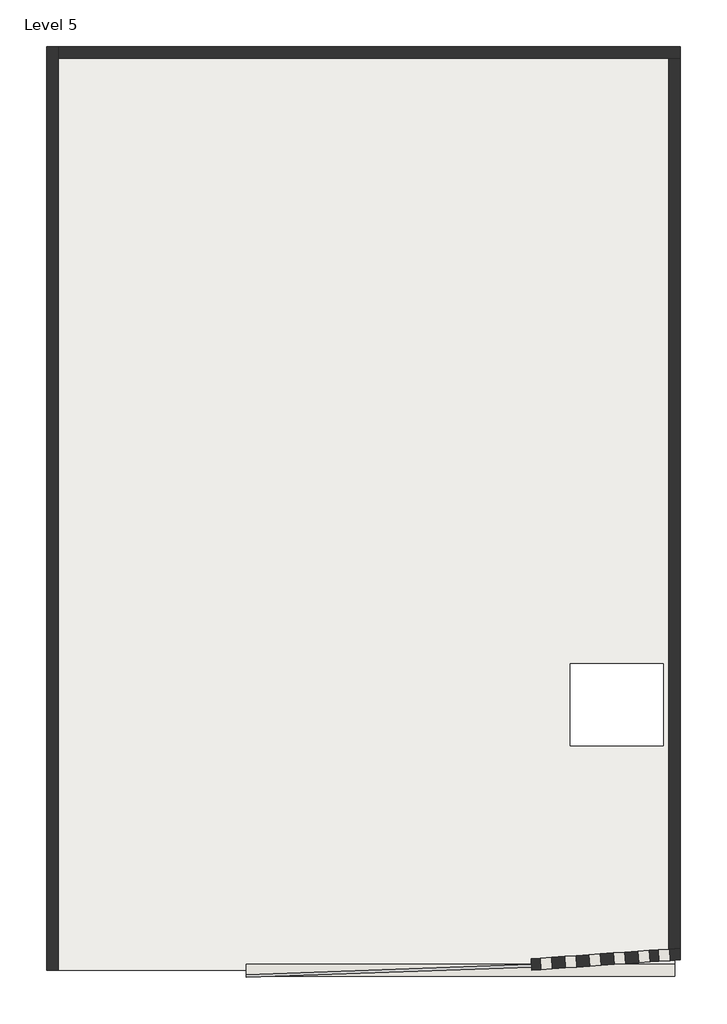
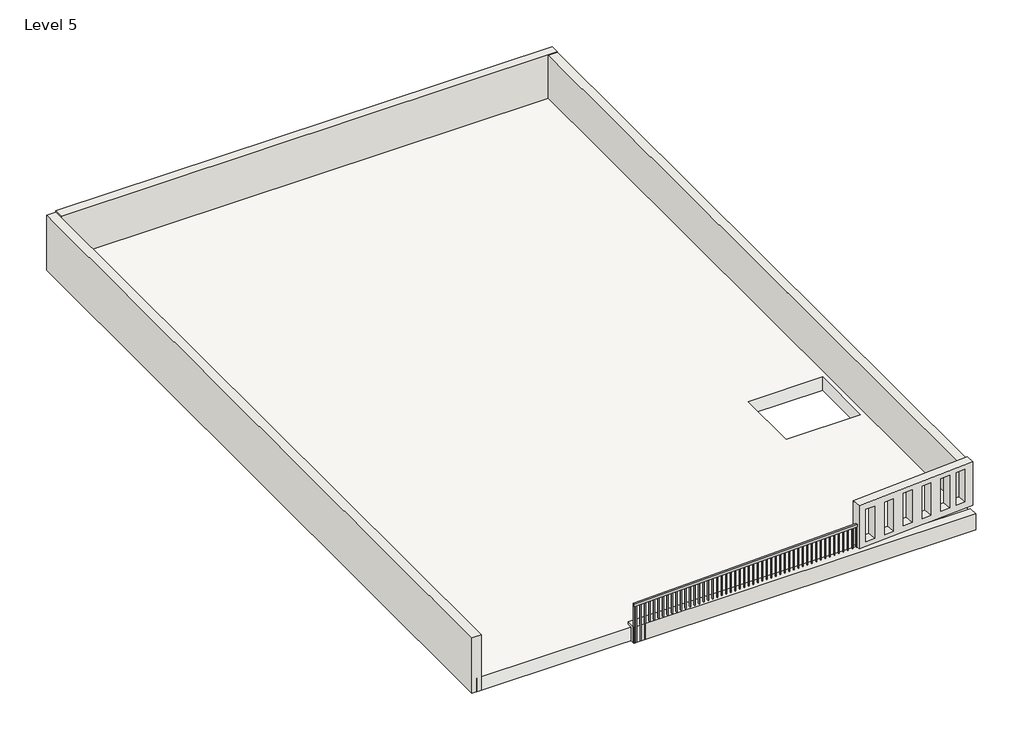
# One storey: 5 walls, 1 railing, 1 roof.
"""IFC4 building model written with IfcOpenShell, lengths in millimetres."""

from ifc_helpers import new_model, si_unit, frame, origin, place, context, project, spatial, polyline, outline, extrude, faceted_brep, element, save

model = new_model("IFC4")

# Units and contexts
model_context = context("Model", 3, world=origin())
ifc_project = project(units=[si_unit("LENGTHUNIT", "METRE", prefix="MILLI")], contexts=[model_context])

# Site, building, storey
site = spatial("IfcSite", under=ifc_project)
building = spatial("IfcBuilding", under=site)
storey = spatial("IfcBuildingStorey", under=building, Name="Level 5", Elevation=12192.0)

# Railing
placement = place(None, origin())
element("IfcRailing", 1, ObjectType="Handrail - Rectangular", at=placement, inside=storey, context=model_context, shape_type="SweptSolid", body=[
    extrude(outline(polyline([(1979.8158974, -8066.6140284), (1981.6116302, -8117.3822797), (-3046.82922, -8295.2441529), (-3048.6249528, -8244.4759015), (1979.8158974, -8066.6140284)])), frame((0.0, 0.0, 13055.6), z_axis=(0.0, 0.0, 1.0), x_axis=(1.0, 0.0, 0.0)), (0.0, 0.0, 1.0), 50.8),
    extrude(outline(polyline([(-2985.3925198, -8258.1242236), (-2984.71912, -8277.1623178), (-3003.7572143, -8277.8357176), (-3004.4306141, -8258.7976234), (-2985.3925198, -8258.1242236)])), frame((0.0, 0.0, 12192.0), z_axis=(0.0, 0.0, 1.0), x_axis=(1.0, 0.0, 0.0)), (0.0, 0.0, 1.0), 863.6),
    extrude(outline(polyline([(-2883.8560172, -8254.5327579), (-2883.1826173, -8273.5708522), (-2902.2207116, -8274.244252), (-2902.8941114, -8255.2061578), (-2883.8560172, -8254.5327579)])), frame((0.0, 0.0, 12192.0), z_axis=(0.0, 0.0, 1.0), x_axis=(1.0, 0.0, 0.0)), (0.0, 0.0, 1.0), 863.6),
    extrude(outline(polyline([(-2782.3195145, -8250.9412923), (-2781.6461147, -8269.9793866), (-2800.6842089, -8270.6527864), (-2801.3576087, -8251.6146921), (-2782.3195145, -8250.9412923)])), frame((0.0, 0.0, 12192.0), z_axis=(0.0, 0.0, 1.0), x_axis=(1.0, 0.0, 0.0)), (0.0, 0.0, 1.0), 863.6),
    extrude(outline(polyline([(-2680.7830118, -8247.3498267), (-2680.109612, -8266.3879209), (-2699.1477063, -8267.0613207), (-2699.8211061, -8248.0232265), (-2680.7830118, -8247.3498267)])), frame((0.0, 0.0, 12192.0), z_axis=(0.0, 0.0, 1.0), x_axis=(1.0, 0.0, 0.0)), (0.0, 0.0, 1.0), 863.6),
    extrude(outline(polyline([(-2579.2465091, -8243.758361), (-2578.5731093, -8262.7964553), (-2597.6112036, -8263.4698551), (-2598.2846034, -8244.4317608), (-2579.2465091, -8243.758361)])), frame((0.0, 0.0, 12192.0), z_axis=(0.0, 0.0, 1.0), x_axis=(1.0, 0.0, 0.0)), (0.0, 0.0, 1.0), 863.6),
    extrude(outline(polyline([(-2477.7100065, -8240.1668954), (-2477.0366067, -8259.2049896), (-2496.0747009, -8259.8783894), (-2496.7481007, -8240.8402952), (-2477.7100065, -8240.1668954)])), frame((0.0, 0.0, 12192.0), z_axis=(0.0, 0.0, 1.0), x_axis=(1.0, 0.0, 0.0)), (0.0, 0.0, 1.0), 863.6),
    extrude(outline(polyline([(-2376.1735038, -8236.5754297), (-2375.500104, -8255.613524), (-2394.5381982, -8256.2869238), (-2395.2115981, -8237.2488295), (-2376.1735038, -8236.5754297)])), frame((0.0, 0.0, 12192.0), z_axis=(0.0, 0.0, 1.0), x_axis=(1.0, 0.0, 0.0)), (0.0, 0.0, 1.0), 863.6),
    extrude(outline(polyline([(-2274.6370011, -8232.9839641), (-2273.9636013, -8252.0220583), (-2293.0016956, -8252.6954581), (-2293.6750954, -8233.6573639), (-2274.6370011, -8232.9839641)])), frame((0.0, 0.0, 12192.0), z_axis=(0.0, 0.0, 1.0), x_axis=(1.0, 0.0, 0.0)), (0.0, 0.0, 1.0), 863.6),
    extrude(outline(polyline([(-2173.1004985, -8229.3924984), (-2172.4270987, -8248.4305927), (-2191.4651929, -8249.1039925), (-2192.1385927, -8230.0658982), (-2173.1004985, -8229.3924984)])), frame((0.0, 0.0, 12192.0), z_axis=(0.0, 0.0, 1.0), x_axis=(1.0, 0.0, 0.0)), (0.0, 0.0, 1.0), 863.6),
    extrude(outline(polyline([(-2071.5639958, -8225.8010328), (-2070.890596, -8244.839127), (-2089.9286902, -8245.5125269), (-2090.60209, -8226.4744326), (-2071.5639958, -8225.8010328)])), frame((0.0, 0.0, 12192.0), z_axis=(0.0, 0.0, 1.0), x_axis=(1.0, 0.0, 0.0)), (0.0, 0.0, 1.0), 863.6),
    extrude(outline(polyline([(-1970.0274931, -8222.2095672), (-1969.3540933, -8241.2476614), (-1988.3921876, -8241.9210612), (-1989.0655874, -8222.882967), (-1970.0274931, -8222.2095672)])), frame((0.0, 0.0, 12192.0), z_axis=(0.0, 0.0, 1.0), x_axis=(1.0, 0.0, 0.0)), (0.0, 0.0, 1.0), 863.6),
    extrude(outline(polyline([(-1868.4909905, -8218.6181015), (-1867.8175906, -8237.6561958), (-1886.8556849, -8238.3295956), (-1887.5290847, -8219.2915013), (-1868.4909905, -8218.6181015)])), frame((0.0, 0.0, 12192.0), z_axis=(0.0, 0.0, 1.0), x_axis=(1.0, 0.0, 0.0)), (0.0, 0.0, 1.0), 863.6),
    extrude(outline(polyline([(-1766.9544878, -8215.0266359), (-1766.281088, -8234.0647301), (-1785.3191822, -8234.7381299), (-1785.992582, -8215.7000357), (-1766.9544878, -8215.0266359)])), frame((0.0, 0.0, 12192.0), z_axis=(0.0, 0.0, 1.0), x_axis=(1.0, 0.0, 0.0)), (0.0, 0.0, 1.0), 863.6),
    extrude(outline(polyline([(-1665.4179851, -8211.4351702), (-1664.7445853, -8230.4732645), (-1683.7826796, -8231.1466643), (-1684.4560794, -8212.10857), (-1665.4179851, -8211.4351702)])), frame((0.0, 0.0, 12192.0), z_axis=(0.0, 0.0, 1.0), x_axis=(1.0, 0.0, 0.0)), (0.0, 0.0, 1.0), 863.6),
    extrude(outline(polyline([(-1563.8814824, -8207.8437046), (-1563.2080826, -8226.8817988), (-1582.2461769, -8227.5551986), (-1582.9195767, -8208.5171044), (-1563.8814824, -8207.8437046)])), frame((0.0, 0.0, 12192.0), z_axis=(0.0, 0.0, 1.0), x_axis=(1.0, 0.0, 0.0)), (0.0, 0.0, 1.0), 863.6),
    extrude(outline(polyline([(-1462.3449798, -8204.2522389), (-1461.67158, -8223.2903332), (-1480.7096742, -8223.963733), (-1481.383074, -8204.9256387), (-1462.3449798, -8204.2522389)])), frame((0.0, 0.0, 12192.0), z_axis=(0.0, 0.0, 1.0), x_axis=(1.0, 0.0, 0.0)), (0.0, 0.0, 1.0), 863.6),
    extrude(outline(polyline([(-1360.8084771, -8200.6607733), (-1360.1350773, -8219.6988675), (-1379.1731715, -8220.3722673), (-1379.8465714, -8201.3341731), (-1360.8084771, -8200.6607733)])), frame((0.0, 0.0, 12192.0), z_axis=(0.0, 0.0, 1.0), x_axis=(1.0, 0.0, 0.0)), (0.0, 0.0, 1.0), 863.6),
    extrude(outline(polyline([(-1259.2719744, -8197.0693076), (-1258.5985746, -8216.1074019), (-1277.6366689, -8216.7808017), (-1278.3100687, -8197.7427075), (-1259.2719744, -8197.0693076)])), frame((0.0, 0.0, 12192.0), z_axis=(0.0, 0.0, 1.0), x_axis=(1.0, 0.0, 0.0)), (0.0, 0.0, 1.0), 863.6),
    extrude(outline(polyline([(-1157.7354718, -8193.477842), (-1157.062072, -8212.5159363), (-1176.1001662, -8213.1893361), (-1176.773566, -8194.1512418), (-1157.7354718, -8193.477842)])), frame((0.0, 0.0, 12192.0), z_axis=(0.0, 0.0, 1.0), x_axis=(1.0, 0.0, 0.0)), (0.0, 0.0, 1.0), 863.6),
    extrude(outline(polyline([(-1056.1989691, -8189.8863764), (-1055.5255693, -8208.9244706), (-1074.5636635, -8209.5978704), (-1075.2370633, -8190.5597762), (-1056.1989691, -8189.8863764)])), frame((0.0, 0.0, 12192.0), z_axis=(0.0, 0.0, 1.0), x_axis=(1.0, 0.0, 0.0)), (0.0, 0.0, 1.0), 863.6),
    extrude(outline(polyline([(-954.6624664, -8186.2949107), (-953.9890666, -8205.333005), (-973.0271609, -8206.0064048), (-973.7005607, -8186.9683105), (-954.6624664, -8186.2949107)])), frame((0.0, 0.0, 12192.0), z_axis=(0.0, 0.0, 1.0), x_axis=(1.0, 0.0, 0.0)), (0.0, 0.0, 1.0), 863.6),
    extrude(outline(polyline([(-853.1259637, -8182.7034451), (-852.4525639, -8201.7415393), (-871.4906582, -8202.4149391), (-872.164058, -8183.3768449), (-853.1259637, -8182.7034451)])), frame((0.0, 0.0, 12192.0), z_axis=(0.0, 0.0, 1.0), x_axis=(1.0, 0.0, 0.0)), (0.0, 0.0, 1.0), 863.6),
    extrude(outline(polyline([(-751.5894611, -8179.1119794), (-750.9160613, -8198.1500737), (-769.9541555, -8198.8234735), (-770.6275553, -8179.7853792), (-751.5894611, -8179.1119794)])), frame((0.0, 0.0, 12192.0), z_axis=(0.0, 0.0, 1.0), x_axis=(1.0, 0.0, 0.0)), (0.0, 0.0, 1.0), 863.6),
    extrude(outline(polyline([(-650.0529584, -8175.5205138), (-649.3795586, -8194.558608), (-668.4176529, -8195.2320078), (-669.0910527, -8176.1939136), (-650.0529584, -8175.5205138)])), frame((0.0, 0.0, 12192.0), z_axis=(0.0, 0.0, 1.0), x_axis=(1.0, 0.0, 0.0)), (0.0, 0.0, 1.0), 863.6),
    extrude(outline(polyline([(-548.5164557, -8171.9290481), (-547.8430559, -8190.9671424), (-566.8811502, -8191.6405422), (-567.55455, -8172.6024479), (-548.5164557, -8171.9290481)])), frame((0.0, 0.0, 12192.0), z_axis=(0.0, 0.0, 1.0), x_axis=(1.0, 0.0, 0.0)), (0.0, 0.0, 1.0), 863.6),
    extrude(outline(polyline([(-446.9799531, -8168.3375825), (-446.3065533, -8187.3756767), (-465.3446475, -8188.0490766), (-466.0180473, -8169.0109823), (-446.9799531, -8168.3375825)])), frame((0.0, 0.0, 12192.0), z_axis=(0.0, 0.0, 1.0), x_axis=(1.0, 0.0, 0.0)), (0.0, 0.0, 1.0), 863.6),
    extrude(outline(polyline([(-345.4434504, -8164.7461169), (-344.7700506, -8183.7842111), (-363.8081448, -8184.4576109), (-364.4815446, -8165.4195167), (-345.4434504, -8164.7461169)])), frame((0.0, 0.0, 12192.0), z_axis=(0.0, 0.0, 1.0), x_axis=(1.0, 0.0, 0.0)), (0.0, 0.0, 1.0), 863.6),
    extrude(outline(polyline([(-243.9069477, -8161.1546512), (-243.2335479, -8180.1927455), (-262.2716422, -8180.8661453), (-262.945042, -8161.828051), (-243.9069477, -8161.1546512)])), frame((0.0, 0.0, 12192.0), z_axis=(0.0, 0.0, 1.0), x_axis=(1.0, 0.0, 0.0)), (0.0, 0.0, 1.0), 863.6),
    extrude(outline(polyline([(-142.3704451, -8157.5631856), (-141.6970452, -8176.6012798), (-160.7351395, -8177.2746796), (-161.4085393, -8158.2365854), (-142.3704451, -8157.5631856)])), frame((0.0, 0.0, 12192.0), z_axis=(0.0, 0.0, 1.0), x_axis=(1.0, 0.0, 0.0)), (0.0, 0.0, 1.0), 863.6),
    extrude(outline(polyline([(-40.8339424, -8153.9717199), (-40.1605426, -8173.0098142), (-59.1986368, -8173.683214), (-59.8720366, -8154.6451197), (-40.8339424, -8153.9717199)])), frame((0.0, 0.0, 12192.0), z_axis=(0.0, 0.0, 1.0), x_axis=(1.0, 0.0, 0.0)), (0.0, 0.0, 1.0), 863.6),
    extrude(outline(polyline([(60.7025603, -8150.3802543), (61.3759601, -8169.4183485), (42.3378658, -8170.0917483), (41.664466, -8151.0536541), (60.7025603, -8150.3802543)])), frame((0.0, 0.0, 12192.0), z_axis=(0.0, 0.0, 1.0), x_axis=(1.0, 0.0, 0.0)), (0.0, 0.0, 1.0), 863.6),
    extrude(outline(polyline([(162.239063, -8146.7887886), (162.9124628, -8165.8268829), (143.8743685, -8166.5002827), (143.2009687, -8147.4621884), (162.239063, -8146.7887886)])), frame((0.0, 0.0, 12192.0), z_axis=(0.0, 0.0, 1.0), x_axis=(1.0, 0.0, 0.0)), (0.0, 0.0, 1.0), 863.6),
    extrude(outline(polyline([(263.7755656, -8143.197323), (264.4489654, -8162.2354172), (245.4108712, -8162.908817), (244.7374714, -8143.8707228), (263.7755656, -8143.197323)])), frame((0.0, 0.0, 12192.0), z_axis=(0.0, 0.0, 1.0), x_axis=(1.0, 0.0, 0.0)), (0.0, 0.0, 1.0), 863.6),
    extrude(outline(polyline([(365.3120683, -8139.6058573), (365.9854681, -8158.6439516), (346.9473739, -8159.3173514), (346.273974, -8140.2792572), (365.3120683, -8139.6058573)])), frame((0.0, 0.0, 12192.0), z_axis=(0.0, 0.0, 1.0), x_axis=(1.0, 0.0, 0.0)), (0.0, 0.0, 1.0), 863.6),
    extrude(outline(polyline([(466.848571, -8136.0143917), (467.5219708, -8155.052486), (448.4838765, -8155.7258858), (447.8104767, -8136.6877915), (466.848571, -8136.0143917)])), frame((0.0, 0.0, 12192.0), z_axis=(0.0, 0.0, 1.0), x_axis=(1.0, 0.0, 0.0)), (0.0, 0.0, 1.0), 863.6),
    extrude(outline(polyline([(568.3850736, -8132.4229261), (569.0584734, -8151.4610203), (550.0203792, -8152.1344201), (549.3469794, -8133.0963259), (568.3850736, -8132.4229261)])), frame((0.0, 0.0, 12192.0), z_axis=(0.0, 0.0, 1.0), x_axis=(1.0, 0.0, 0.0)), (0.0, 0.0, 1.0), 863.6),
    extrude(outline(polyline([(669.9215763, -8128.8314604), (670.5949761, -8147.8695547), (651.5568819, -8148.5429545), (650.8834821, -8129.5048602), (669.9215763, -8128.8314604)])), frame((0.0, 0.0, 12192.0), z_axis=(0.0, 0.0, 1.0), x_axis=(1.0, 0.0, 0.0)), (0.0, 0.0, 1.0), 863.6),
    extrude(outline(polyline([(771.458079, -8125.2399948), (772.1314788, -8144.278089), (753.0933845, -8144.9514888), (752.4199847, -8125.9133946), (771.458079, -8125.2399948)])), frame((0.0, 0.0, 12192.0), z_axis=(0.0, 0.0, 1.0), x_axis=(1.0, 0.0, 0.0)), (0.0, 0.0, 1.0), 863.6),
    extrude(outline(polyline([(872.9945816, -8121.6485291), (873.6679815, -8140.6866234), (854.6298872, -8141.3600232), (853.9564874, -8122.3219289), (872.9945816, -8121.6485291)])), frame((0.0, 0.0, 12192.0), z_axis=(0.0, 0.0, 1.0), x_axis=(1.0, 0.0, 0.0)), (0.0, 0.0, 1.0), 863.6),
    extrude(outline(polyline([(974.5310843, -8118.0570635), (975.2044841, -8137.0951577), (956.1663899, -8137.7685575), (955.4929901, -8118.7304633), (974.5310843, -8118.0570635)])), frame((0.0, 0.0, 12192.0), z_axis=(0.0, 0.0, 1.0), x_axis=(1.0, 0.0, 0.0)), (0.0, 0.0, 1.0), 863.6),
    extrude(outline(polyline([(1076.067587, -8114.4655978), (1076.7409868, -8133.5036921), (1057.7028925, -8134.1770919), (1057.0294927, -8115.1389976), (1076.067587, -8114.4655978)])), frame((0.0, 0.0, 12192.0), z_axis=(0.0, 0.0, 1.0), x_axis=(1.0, 0.0, 0.0)), (0.0, 0.0, 1.0), 863.6),
    extrude(outline(polyline([(1177.6040897, -8110.8741322), (1178.2774895, -8129.9122264), (1159.2393952, -8130.5856263), (1158.5659954, -8111.547532), (1177.6040897, -8110.8741322)])), frame((0.0, 0.0, 12192.0), z_axis=(0.0, 0.0, 1.0), x_axis=(1.0, 0.0, 0.0)), (0.0, 0.0, 1.0), 863.6),
    extrude(outline(polyline([(1279.1405923, -8107.2826666), (1279.8139921, -8126.3207608), (1260.7758979, -8126.9941606), (1260.1024981, -8107.9560664), (1279.1405923, -8107.2826666)])), frame((0.0, 0.0, 12192.0), z_axis=(0.0, 0.0, 1.0), x_axis=(1.0, 0.0, 0.0)), (0.0, 0.0, 1.0), 863.6),
    extrude(outline(polyline([(1380.677095, -8103.6912009), (1381.3504948, -8122.7292952), (1362.3124006, -8123.402695), (1361.6390007, -8104.3646007), (1380.677095, -8103.6912009)])), frame((0.0, 0.0, 12192.0), z_axis=(0.0, 0.0, 1.0), x_axis=(1.0, 0.0, 0.0)), (0.0, 0.0, 1.0), 863.6),
    extrude(outline(polyline([(1482.2135977, -8100.0997353), (1482.8869975, -8119.1378295), (1463.8489032, -8119.8112293), (1463.1755034, -8100.7731351), (1482.2135977, -8100.0997353)])), frame((0.0, 0.0, 12192.0), z_axis=(0.0, 0.0, 1.0), x_axis=(1.0, 0.0, 0.0)), (0.0, 0.0, 1.0), 863.6),
    extrude(outline(polyline([(1583.7501003, -8096.5082696), (1584.4235001, -8115.5463639), (1565.3854059, -8116.2197637), (1564.7120061, -8097.1816694), (1583.7501003, -8096.5082696)])), frame((0.0, 0.0, 12192.0), z_axis=(0.0, 0.0, 1.0), x_axis=(1.0, 0.0, 0.0)), (0.0, 0.0, 1.0), 863.6),
    extrude(outline(polyline([(1685.286603, -8092.916804), (1685.9600028, -8111.9548982), (1666.9219086, -8112.628298), (1666.2485088, -8093.5902038), (1685.286603, -8092.916804)])), frame((0.0, 0.0, 12192.0), z_axis=(0.0, 0.0, 1.0), x_axis=(1.0, 0.0, 0.0)), (0.0, 0.0, 1.0), 863.6),
    extrude(outline(polyline([(1786.8231057, -8089.3253383), (1787.4965055, -8108.3634326), (1768.4584112, -8109.0368324), (1767.7850114, -8089.9987381), (1786.8231057, -8089.3253383)])), frame((0.0, 0.0, 12192.0), z_axis=(0.0, 0.0, 1.0), x_axis=(1.0, 0.0, 0.0)), (0.0, 0.0, 1.0), 863.6),
    extrude(outline(polyline([(1888.3596084, -8085.7338727), (1889.0330082, -8104.7719669), (1869.9949139, -8105.4453667), (1869.3215141, -8086.4072725), (1888.3596084, -8085.7338727)])), frame((0.0, 0.0, 12192.0), z_axis=(0.0, 0.0, 1.0), x_axis=(1.0, 0.0, 0.0)), (0.0, 0.0, 1.0), 863.6),
    extrude(outline(polyline([(-3029.025692, -8259.6675803), (-3028.3522922, -8278.7056745), (-3047.3903865, -8279.3790743), (-3048.0637863, -8260.3409801), (-3029.025692, -8259.6675803)])), frame((0.0, 0.0, 12192.0), z_axis=(0.0, 0.0, 1.0), x_axis=(1.0, 0.0, 0.0)), (0.0, 0.0, 1.0), 863.6),
    extrude(outline(polyline([(1980.3770639, -8082.4791069), (1981.0504637, -8101.5172012), (1962.0123695, -8102.190601), (1961.3389696, -8083.1525068), (1980.3770639, -8082.4791069)])), frame((0.0, 0.0, 12192.0), z_axis=(0.0, 0.0, 1.0), x_axis=(1.0, 0.0, 0.0)), (0.0, 0.0, 1.0), 863.6),
])

# Roof
element("IfcRoof", 2, ObjectType="Generic - 12\"", at=placement, inside=storey, context=model_context, shape_type="SweptSolid", body=[
    extrude(outline(polyline([(-6461.1108866, -8168.2600272), (-6461.1108866, 7998.8399728), (4498.9891134, 7998.8399728), (4498.9891134, -8168.2600272), (-6461.1108866, -8168.2600272)]), holes=[polyline([(4295.7891134, -2770.7600272), (2657.4891134, -2770.7600272), (2657.4891134, -4218.5600272), (4295.7891134, -4218.5600272), (4295.7891134, -2770.7600272)])]), frame((0.0, 0.0, 12192.0), z_axis=(0.0, 0.0, 1.0), x_axis=(1.0, 0.0, 0.0)), (0.0, 0.0, 1.0), 304.8),
])

# Walls
element("IfcWall", 3, ObjectType="9\" w", at=placement, inside=storey, context=model_context, shape_type="SweptSolid", body=[
    extrude(outline(polyline([(4498.9891134, -8269.8600272), (-3047.7270864, -8269.8600272), (-3047.7270864, -8066.6600272), (4498.9891134, -8066.6600272), (4498.9891134, -8269.8600272)])), frame((0.0, 0.0, 12192.0), z_axis=(0.0, 0.0, 1.0), x_axis=(1.0, 0.0, 0.0)), (0.0, 0.0, 1.0), 370.4907484),
])
element("IfcWall", 4, ObjectType="9\" w", at=placement, inside=storey, context=model_context, shape_type="Brep", body=[
    faceted_brep([(1986.0292071, -8168.0125347, 12562.4907484), (4600.5891134, -7985.1846958, 12562.4907484), (4600.5891134, -7985.1846958, 13570.9676266), (1986.0292071, -8168.0125347, 13570.9676266), (2347.8973793, -8142.7082471, 13423.9934861), (2347.8973793, -8142.7082471, 12666.5569695), (2145.1923643, -8156.8827625, 12666.5569695), (2145.1923643, -8156.8827625, 13423.9934861), (2778.6455362, -8112.5874017, 13423.9934861), (2778.6455362, -8112.5874017, 12666.5569695), (2575.9405212, -8126.7619172, 12666.5569695), (2575.9405212, -8126.7619172, 13423.9934861), (3207.7545663, -8082.5811753, 13461.6273358), (3207.7545663, -8082.5811753, 12704.1908192), (3005.0495513, -8096.7556907, 12704.1908192), (3005.0495513, -8096.7556907, 13461.6273358), (3638.5027232, -8052.4603299, 13461.6273358), (3638.5027232, -8052.4603299, 12704.1908192), (3435.7977082, -8066.6348454, 12704.1908192), (3435.7977082, -8066.6348454, 13461.6273358), (4069.2508801, -8022.3394845, 13461.6273358), (4069.2508801, -8022.3394845, 12704.1908192), (3866.5458651, -8036.514, 12704.1908192), (3866.5458651, -8036.514, 13461.6273358), (4423.9846564, -7997.5340825, 13461.6273358), (4423.9846564, -7997.5340825, 12704.1908192), (4221.2796414, -8011.7085979, 12704.1908192), (4221.2796414, -8011.7085979, 13461.6273358), (1971.8546916, -7965.3075197, 12562.4907484), (1971.8546916, -7965.3075197, 13570.9676266), (4600.5891134, -7781.4885021, 13570.9676266), (4600.5891134, -7781.4885021, 13502.8084917), (4600.5891134, -7781.4885021, 12562.4907484), (2333.7228638, -7940.0032321, 13423.9934861), (2131.0178488, -7954.1777475, 13423.9934861), (2131.0178488, -7954.1777475, 12666.5569695), (2333.7228638, -7940.0032321, 12666.5569695), (2764.4710207, -7909.8823867, 13423.9934861), (2561.7660057, -7924.0569022, 13423.9934861), (2561.7660057, -7924.0569022, 12666.5569695), (2764.4710207, -7909.8823867, 12666.5569695), (3193.5800508, -7879.8761603, 13461.6273358), (2990.8750358, -7894.0506757, 13461.6273358), (2990.8750358, -7894.0506757, 12704.1908192), (3193.5800508, -7879.8761603, 12704.1908192), (3624.3282077, -7849.7553149, 13461.6273358), (3421.6231927, -7863.9298304, 13461.6273358), (3421.6231927, -7863.9298304, 12704.1908192), (3624.3282077, -7849.7553149, 12704.1908192), (4055.0763646, -7819.6344695, 13461.6273358), (3852.3713496, -7833.808985, 13461.6273358), (3852.3713496, -7833.808985, 12704.1908192), (4055.0763646, -7819.6344695, 12704.1908192), (4409.8101409, -7794.8290675, 13461.6273358), (4207.1051259, -7809.0035829, 13461.6273358), (4207.1051259, -7809.0035829, 12704.1908192), (4409.8101409, -7794.8290675, 12704.1908192)], [[[0, 1, 2, 3], [4, 5, 6, 7], [8, 9, 10, 11], [12, 13, 14, 15], [16, 17, 18, 19], [20, 21, 22, 23], [24, 25, 26, 27]], [[28, 29, 30, 31, 32], [33, 34, 35, 36], [37, 38, 39, 40], [41, 42, 43, 44], [45, 46, 47, 48], [49, 50, 51, 52], [53, 54, 55, 56]], [[1, 0, 28, 32]], [[3, 2, 30, 29]], [[0, 3, 29, 28]], [[5, 4, 33, 36]], [[6, 5, 36, 35]], [[7, 6, 35, 34]], [[4, 7, 34, 33]], [[9, 8, 37, 40]], [[10, 9, 40, 39]], [[11, 10, 39, 38]], [[8, 11, 38, 37]], [[13, 12, 41, 44]], [[14, 13, 44, 43]], [[15, 14, 43, 42]], [[12, 15, 42, 41]], [[17, 16, 45, 48]], [[18, 17, 48, 47]], [[19, 18, 47, 46]], [[16, 19, 46, 45]], [[21, 20, 49, 52]], [[22, 21, 52, 51]], [[23, 22, 51, 50]], [[20, 23, 50, 49]], [[25, 24, 53, 56]], [[26, 25, 56, 55]], [[27, 26, 55, 54]], [[24, 27, 54, 53]], [[2, 1, 32, 31, 30]]]),
])
element("IfcWall", 5, ObjectType="9\" w", at=placement, inside=storey, context=model_context, shape_type="Brep", body=[
    faceted_brep([(-6359.5108866, -8168.2600272, 12192.0), (-6359.5108866, 7897.2399728, 12192.0), (-6359.5108866, 8100.4399728, 12192.0), (-6359.5108866, 8100.4399728, 13486.1036122), (-6359.5108866, -8168.2600272, 13486.1036122), (-6562.7108866, -8168.2600272, 12192.0), (-6562.7108866, -8168.2600272, 13486.1036122), (-6562.7108866, 8100.4399728, 13486.1036122), (-6562.7108866, 8100.4399728, 12192.0)], [[[0, 1, 2, 3, 4]], [[5, 6, 7, 8]], [[2, 1, 0, 5, 8]], [[4, 3, 7, 6]], [[0, 4, 6, 5]], [[3, 2, 8, 7]]]),
])
element("IfcWall", 6, ObjectType="9\" w", at=placement, inside=storey, context=model_context, shape_type="Brep", body=[
    faceted_brep([(-6359.5108866, 7897.2399728, 12192.0), (4397.3891134, 7897.2399728, 12192.0), (4600.5891134, 7897.2399728, 12192.0), (4600.5891134, 7897.2399728, 13502.8084917), (4600.5891134, 7897.2399728, 13511.7599199), (-6359.5108866, 7897.2399728, 13511.7599199), (-6359.5108866, 8100.4399728, 12192.0), (-6359.5108866, 8100.4399728, 13486.1036122), (-6359.5108866, 8100.4399728, 13511.7599199), (4600.5891134, 8100.4399728, 13511.7599199), (4600.5891134, 8100.4399728, 12192.0)], [[[0, 1, 2, 3, 4, 5]], [[6, 7, 8, 9, 10]], [[2, 1, 0, 6, 10]], [[5, 4, 9, 8]], [[0, 5, 8, 7, 6]], [[4, 3, 2, 10, 9]]]),
])
element("IfcWall", 7, ObjectType="9\" w", at=placement, inside=storey, context=model_context, shape_type="Brep", body=[
    faceted_brep([(4397.3891134, 7897.2399728, 12192.0), (4397.3891134, -7795.6976303, 12192.0), (4397.3891134, -7795.6976303, 13502.8084917), (4397.3891134, 7897.2399728, 13502.8084917), (4600.5891134, 7897.2399728, 12192.0), (4600.5891134, 7897.2399728, 13502.8084917), (4600.5891134, -7781.4885021, 13502.8084917), (4600.5891134, -7781.4885021, 12562.4907484), (4600.5891134, -7781.4885021, 12192.0)], [[[0, 1, 2, 3]], [[4, 5, 6, 7, 8]], [[1, 0, 4, 8]], [[3, 2, 6, 5]], [[0, 3, 5, 4]], [[1, 8, 7, 6, 2]]]),
])

save(model, "model.ifc")

# Revit data of these elements
# Type "Handrail - Rectangular"
#   Assembly Code = "C2010400"
#   built-in parameter 1008612 = 0.0416667 (stored number, unit not read)
#   built-in parameter 1008611 = 0.0416667 (stored number, unit not read)
#   built-in parameter 1008609 = 0.333333 (stored number, unit not read)
#   built-in parameter 1008604 = 0.166667 (stored number, unit not read)
#   built-in parameter 1008603 = 0.166667 (stored number, unit not read)
#   Railing Height = 3' - 0"
#   built-in parameter 1008630 = 2
#   built-in parameter 1008610 = 2
#   built-in parameter 1008618 = Baluster - Square : 3/4"
# Type "Generic - 12\""
#   Assembly Code = "B1020"
#   Layers, outside or top first: 1' - 0" no material (function 1)
# Type "9\" w"
#   Assembly Code = "B2010"
#   Layers, outside or top first: 0' - 8" no material (function 1)
# Element 1 (IfcRailing, "Handrail - Rectangular")
#   Phase Created = New Construction
#   Materials on its faces: "Iron, Ductile"
# Element 2 (IfcRoof, "Generic - 12\"")
#   built-in parameter 1001705 = 41 (stored number, unit not read)
#   built-in parameter 1001710 = 33615
#   Phase Created = New Construction
#   Materials on its faces: "Default Roof", "Window Frame", "Earth", "Vapor Retarder"
# Element 3 (IfcWall, "9\" w")
#   Top Offset = 0' - 0"
#   Base Offset = 0' - 0"
#   Unconnected Height = 1' - 2.58625"
#   wall height = 1' - 2.58625"
#   Phase Created = New Construction
#   Base Constraint = Level 5
#   Materials on its faces: "Default Wall", "Doors - Glazing Bars"
# Element 4 (IfcWall, "9\" w")
#   built-in parameter 1001111 = 1' - 2.58625"
#   Top Offset = 0' - 0"
#   Base Offset = 1' - 2.58625"
#   Unconnected Height = 3' - 3.70381"
#   wall height = 3' - 3.70381"
#   Phase Created = New Construction
#   Base Constraint = Level 5
#   Materials on its faces: "Default Wall", "Doors - Glazing Bars", "Oak Flooring"
# Element 5 (IfcWall, "9\" w")
#   Top Offset = 0' - 0"
#   Base Offset = 0' - 0"
#   Unconnected Height = 4' - 2.94896"
#   wall height = 4' - 2.94896"
#   Phase Created = New Construction
#   Base Constraint = Level 5
#   Materials on its faces: "Doors - Glazing Bars", "Default Wall"
# Element 6 (IfcWall, "9\" w")
#   Top Offset = 0' - 0"
#   Base Offset = 0' - 0"
#   Unconnected Height = 4' - 3.95905"
#   wall height = 4' - 3.95905"
#   Phase Created = New Construction
#   Base Constraint = Level 5
#   Materials on its faces: "Doors - Glazing Bars", "Default Wall"
# Element 7 (IfcWall, "9\" w")
#   Top Offset = 0' - 0"
#   Base Offset = 0' - 0"
#   Unconnected Height = 4' - 3.60663"
#   wall height = 4' - 3.60663"
#   Phase Created = New Construction
#   Base Constraint = Level 5
#   Materials on its faces: "Doors - Glazing Bars", "Default Wall"
# Materials
#   "Iron, Ductile": class "Metal", colour RGB 0 0 0, transparency 0, Description = "Ductile cast iron", Cost = 0
#   "Default Roof": colour RGB 88 101 114, transparency 0, Cost = 0
#   "Window Frame": colour RGB 249 249 249, transparency 0
#   "Earth": class "Generic", colour RGB 97 75 62, transparency 0, Description = "Soil", Cost = 0
#   "Vapor Retarder": class "Generic", colour RGB 127 127 127, transparency 0, Description = "Polyethylene film membrane", Cost = 0
#   "Default Wall": colour RGB 128 128 128, transparency 0, Cost = 0
#   "Doors - Glazing Bars": colour RGB 158 107 65, transparency 0
#   "Oak Flooring": class "Wood", colour RGB 216 169 114, transparency 0, Description = "Quercus Rubra", Cost = 0
